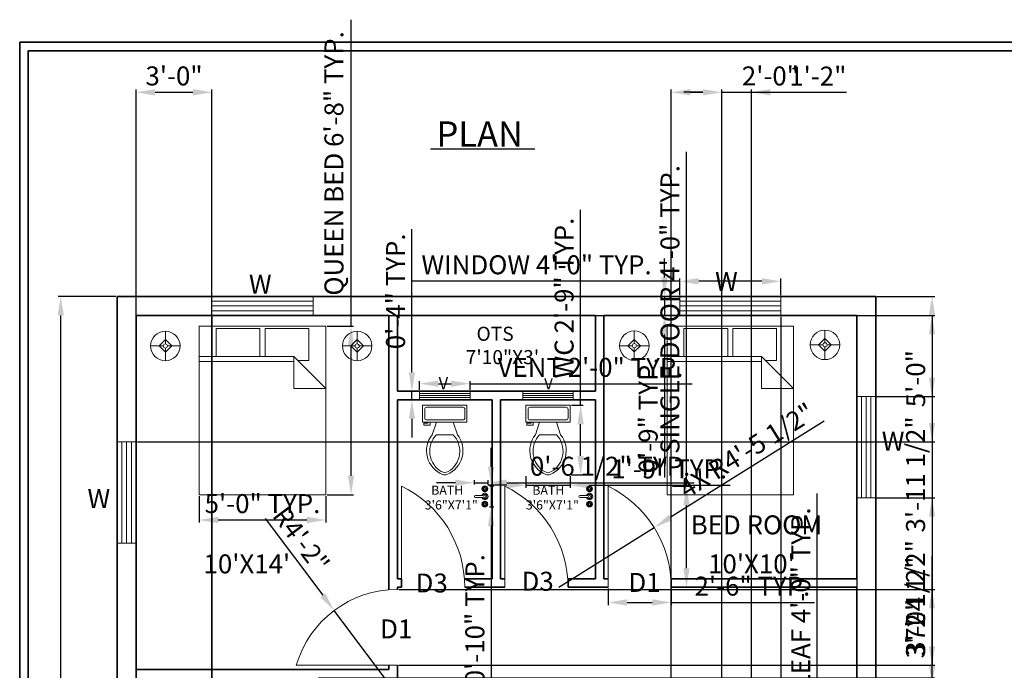
# Model space of a CAD drawing. Units: inches. Extents: x 2436 to 3928, y 1526 to 2149.
# Tile 4 of 6: x 2436 to 2903, y 1840 to 2149. Entities that reach past the tile are written whole.
import ezdxf

# ---------------------------------------------------------------- set-up
doc = ezdxf.new("R2010")
doc.units = ezdxf.units.IN
for name, color, linetype, lineweight in [('A-AREA-IDEN', 152, 'Continuous', 18), ('A-DOOR', 4, 'Continuous', 18), ('A-DOOR-TEXT', 30, 'Continuous', 18), ('A-FLOR-FIXT', 9, 'Continuous', 18), ('A-FURN', 8, 'Continuous', 18), ('A-GLAZ', 2, 'Continuous', 18), ('A-GLAZ-TEXT', 114, 'Continuous', 18), ('A-WALL', 7, 'Continuous', 35), ('G-ANNO-TEXT', 7, 'Continuous', 25), ('G-ANNO-TTLB', 7, 'Continuous', 35), ('S-ANNO-DIMS', 2, 'Continuous', 18)]:
    doc.layers.add(name, color=color, linetype=linetype, lineweight=lineweight)
doc.styles.get("Standard").update_dxf_attribs({"font": 'arial.ttf'})
doc.dimstyles.new('ISO-25', dxfattribs={"dimtxt": 9, "dimasz": 9, "dimexe": 1.25, "dimexo": 0.625, "dimgap": 2, "dimtad": 1, "dimdec": 1, "dimlunit": 4, "dimtxsty": 'Standard', "dimcen": 2.5, "dimadec": 0, "dimazin": 0, "dimtfac": 1, "dimtdec": 1, "dimtmove": 0, "dimatfit": 3, "dimfxl": 1, "dimarcsym": 0})

# ---------------------------------------------------------------- blocks, each defined once
blk = doc.blocks.new('Bed - Queen')
for p, q in [((0, -80.00003), (0, 0)), ((0, 0), (59.99999, 0)), ((59.99999, 0), (59.99999, -80.00003)), ((7.99999, -1.2), (28.79998, -1.2)), ((7.99999, -14.4), (7.99999, -1.2)), ((28.79998, -1.2), (28.79998, -14.4)), ((31.19999, -1.2), (51.99999, -1.2)), ((31.19999, -14.4), (31.19999, -1.2)), ((51.99999, -1.2), (51.99999, -16.4)), ((0, -14.4), (44.8, -14.4)), ((44.8, -16.8), (0, -16.8)), ((59.99999, -29.6), (44.8, -14.4)), ((44.8, -14.4), (44.8, -29.6)), ((51.99999, -16.4), (46.79936, -16.4)), ((44.8, -29.6), (59.99999, -29.6)), ((59.99999, -80.00003), (0, -80.00003))]:
    blk.add_line(p, q)
blk = doc.blocks.new('Toilet - top')
for p, q in [((9.5, -6), (9.5, -2)), ((-10, -8.5), (-8, -8.5)), ((-10, -9.5), (-10, -8.5)), ((-8, -8.5), (-8, -8)), ((-7, -8), (-7, -9.5)), ((-4, -8), (-6, -14)), ((4, -8), (6, -14)), ((-7, -9.5), (-10, -9.5)), ((4, -14), (-4, -14))]:
    blk.add_line(p, q)
blk.add_lwpolyline([(10.5, -8), (10.5, 0), (-10.5, 0), (-10.5, -8)], close=True)
for points in [[(-9.5, -2), (-9.5, -6)], [(8.5, -1), (-8.5, -1)], [(-8.5, -7), (8.5, -7)]]:
    blk.add_lwpolyline(points)
for centre, radius, start, end in [((-8.62, -1.88), 0.884, 81.8699, 188.1301), ((8.62, -1.88), 0.884, 351.8699, 98.1301), ((-8.62, -6.12), 0.884, 171.8699, 278.1301), ((8.62, -6.12), 0.884, 261.8699, 8.1301), ((3.52, -21.58), 12.17, 141.4691, 247.9714), ((4.2, -21.82), 11.33, 136.3677, 238.9468), ((-3.52, -21.58), 12.17, 292.0284, 38.5307), ((-4.2, -21.82), 11.33, 301.053, 43.6321), ((0, -27.88), 4, 245.7318, 294.2682), ((0, -29), 4, 254.8605, 285.1395)]:
    blk.add_arc(centre, radius, start, end)
blk = doc.blocks.new('Faucet - Bathroom top')
for p, q in [((-4.107, 0.125), (-4.375, 0.125)), ((-3.75, 0.4788), (-3.75, 0.75)), ((-3.5, 0.482), (-3.5, 0.75)), ((-3.1461, 0.125), (-2.875, 0.125)), ((3.143, 0.125), (2.875, 0.125)), ((3.5, 0.4788), (3.5, 0.75)), ((3.75, 0.482), (3.75, 0.75)), ((4.1039, 0.125), (4.375, 0.125)), ((-4.1039, -0.125), (-4.375, -0.125)), ((-3.75, -0.4821), (-3.75, -0.75)), ((-3.5, -0.4789), (-3.5, -0.75)), ((-3.143, -0.125), (-2.875, -0.125)), ((-0.5, -0.8639), (-0.5, -4.5)), ((0.5, -4.5), (0.5, -0.8631)), ((3.1461, -0.125), (2.875, -0.125)), ((3.5, -0.4821), (3.5, -0.75)), ((3.75, -0.4789), (3.75, -0.75)), ((4.107, -0.125), (4.375, -0.125))]:
    blk.add_line(p, q)
for centre, radius in [((-3.625, 0), 1.375), ((-4.625, 0), 0.2795), ((-3.625, 0), 0.5), ((-3.625, 1), 0.2795), ((-2.625, 0), 0.2795), ((0, 0), 0.5), ((3.625, 0), 1.375), ((2.625, 0), 0.2795), ((3.625, 0), 0.5), ((3.625, 1), 0.2795), ((4.625, 0), 0.2795), ((-3.625, -1), 0.2795), ((3.625, -1), 0.2795)]:
    blk.add_circle(centre, radius)
for centre, radius, start, end in [((-3.625, 0), 1, 105.2407, 164.2093), ((-3.625, 0), 1, 16.44125, 74.07887), ((0, 0), 1.5, 289.6514, 250.3603), ((0, 0), 1, 300.3431, 239.7554), ((3.625, 0), 1, 106.12, 164.0884), ((3.625, 0), 1, 16.23422, 73.90469), ((-3.625, 0), 1, 196.2342, 253.9047), ((-3.625, 0), 1, 286.12, 344.0884), ((0, -4.5), 0.5, 180, 0), ((3.625, 0), 1, 196.4413, 254.0789), ((3.625, 0), 1, 285.2407, 344.2093)]:
    blk.add_arc(centre, radius, start, end)
blk = doc.blocks.new('Lamp - Table')
for p, q in [((0, 7), (0, 1)), ((-1, 0), (-7, 0)), ((0, 3), (-3, 0)), ((-3, 0), (0, -3)), ((3, 0), (0, 3)), ((0, -3), (3, 0)), ((1, 0), (7, 0)), ((0, -1), (0, -7))]:
    blk.add_line(p, q)
for radius in [7, 1]:
    blk.add_circle((0, 0), radius)
blk = doc.blocks.new('WIN-48x9-PLAN')
for p, q in [((0, 0), (0, 9)), ((0, 6.75), (48, 6.75)), ((48, 0), (48, 9)), ((0, 4.5), (48, 4.5)), ((0, 2.25), (48, 2.25))]:
    blk.add_line(p, q)
blk = doc.blocks.new('VENT-24x4-PLAN')
for p, q in [((0, 0), (0, 4)), ((0, 3), (24, 3)), ((0, 2), (24, 2)), ((0, 1), (24, 1)), ((24, 0), (24, 4))]:
    blk.add_line(p, q)
blk = doc.blocks.new('DOOR-SINGLE-30-PLAN')
blk.add_line((0, 0), (0, 48))
blk.add_arc((-23.4, 0), 53.4, 0, 64.0108)
blk = doc.blocks.new('*D34')
at = {"layer": 'Defpoints', "color": 0, "transparency": 16777216}
for p in [(2749.24, 2024.99), (2749.24, 2017.79), (2797.24, 2017.79)]:
    blk.add_point(p, dxfattribs=at)
at = {"layer": 'S-ANNO-DIMS', "color": 0, "lineweight": -2, "transparency": 16777216}
for p, q in [((2749.24, 2024.99), (2622.35, 2024.99)), ((2749.24, 2018.41), (2749.24, 2026.24)), ((2788.24, 2024.99), (2758.24, 2024.99)), ((2797.24, 2018.41), (2797.24, 2026.24))]:
    blk.add_line(p, q, dxfattribs=at)
at = {"layer": 'S-ANNO-DIMS', "color": 0, "transparency": 16777216}
for points in [[(2758.24, 2026.49), (2758.24, 2023.49), (2749.24, 2024.99)], [(2788.24, 2026.49), (2788.24, 2023.49), (2797.24, 2024.99)]]:
    blk.add_solid(points, dxfattribs=at)
at = {"layer": 'S-ANNO-DIMS', "color": 0, "transparency": 16777216, "insert": (2681.29, 2031.65), "char_height": 9, "attachment_point": 5}
blk.add_mtext('WINDOW 4\'-0" TYP.', dxfattribs=at)
blk = doc.blocks.new('*D35')
at = {"layer": 'Defpoints', "color": 0, "transparency": 16777216}
for p in [(2749.24, 2017.79), (2742.04, 2008.79), (2749.24, 2008.79)]:
    blk.add_point(p, dxfattribs=at)
at = {"layer": 'S-ANNO-DIMS', "color": 0, "lineweight": -2, "transparency": 16777216}
for p, q in [((2742.04, 2026.79), (2742.04, 2035.79)), ((2748.61, 2017.79), (2740.79, 2017.79)), ((2742.04, 2017.79), (2742.04, 2008.79)), ((2748.61, 2008.79), (2740.79, 2008.79)), ((2742.04, 1999.79), (2742.04, 1931.93))]:
    blk.add_line(p, q, dxfattribs=at)
at = {"layer": 'S-ANNO-DIMS', "color": 0, "transparency": 16777216}
for points in [[(2740.54, 2026.79), (2743.54, 2026.79), (2742.04, 2017.79)], [(2740.54, 1999.79), (2743.54, 1999.79), (2742.04, 2008.79)]]:
    blk.add_solid(points, dxfattribs=at)
at = {"layer": 'S-ANNO-DIMS', "color": 0, "transparency": 16777216, "insert": (2735.44, 1961.36), "char_height": 9, "attachment_point": 5, "rotation": 90}
blk.add_mtext('0\'-9" TYP.', dxfattribs=at)
blk = doc.blocks.new('*D36')
at = {"layer": 'Defpoints', "color": 0, "transparency": 16777216}
for p in [(2745.24, 1927.79), (2752.44, 1927.79), (2745.24, 1879.79)]:
    blk.add_point(p, dxfattribs=at)
at = {"layer": 'S-ANNO-DIMS', "color": 0, "lineweight": -2, "transparency": 16777216}
for p, q in [((2752.44, 1927.79), (2752.44, 2086.43)), ((2745.86, 1927.79), (2753.69, 1927.79)), ((2752.44, 1888.79), (2752.44, 1918.79)), ((2745.86, 1879.79), (2753.69, 1879.79))]:
    blk.add_line(p, q, dxfattribs=at)
at = {"layer": 'S-ANNO-DIMS', "color": 0, "transparency": 16777216}
for points in [[(2750.94, 1918.79), (2753.94, 1918.79), (2752.44, 1927.79)], [(2750.94, 1888.79), (2753.94, 1888.79), (2752.44, 1879.79)]]:
    blk.add_solid(points, dxfattribs=at)
at = {"layer": 'S-ANNO-DIMS', "color": 0, "transparency": 16777216, "insert": (2745.78, 2011.61), "char_height": 9, "attachment_point": 5, "rotation": 90}
blk.add_mtext('SINGLE DOOR 4\'-0" TYP.', dxfattribs=at)
blk = doc.blocks.new('*D37')
at = {"layer": 'Defpoints', "color": 0, "transparency": 16777216}
for p in [(2715.24, 1879.79), (2745.24, 1879.79), (2745.24, 1872.59)]:
    blk.add_point(p, dxfattribs=at)
at = {"layer": 'S-ANNO-DIMS', "color": 0, "lineweight": -2, "transparency": 16777216}
for p, q in [((2715.24, 1879.16), (2715.24, 1871.34)), ((2745.24, 1879.16), (2745.24, 1871.34)), ((2724.24, 1872.59), (2736.24, 1872.59)), ((2745.24, 1872.59), (2813.25, 1872.59))]:
    blk.add_line(p, q, dxfattribs=at)
at = {"layer": 'S-ANNO-DIMS', "color": 0, "transparency": 16777216}
for points in [[(2724.24, 1874.09), (2724.24, 1871.09), (2715.24, 1872.59)], [(2736.24, 1874.09), (2736.24, 1871.09), (2745.24, 1872.59)]]:
    blk.add_solid(points, dxfattribs=at)
at = {"layer": 'S-ANNO-DIMS', "color": 0, "transparency": 16777216, "insert": (2783.74, 1879.18), "char_height": 9, "attachment_point": 5}
blk.add_mtext('2\'-6" TYP.', dxfattribs=at)
blk = doc.blocks.new('*D38')
at = {"layer": 'Defpoints', "color": 0, "transparency": 16777216}
for p in [(2581.24, 2003.73), (2593.24, 2003.73), (2581.24, 1923.73)]:
    blk.add_point(p, dxfattribs=at)
at = {"layer": 'S-ANNO-DIMS', "color": 0, "lineweight": -2, "transparency": 16777216}
for p, q in [((2593.24, 2003.73), (2593.24, 2149.12)), ((2581.86, 2003.73), (2594.49, 2003.73)), ((2593.24, 1932.73), (2593.24, 1994.73)), ((2581.86, 1923.73), (2594.49, 1923.73))]:
    blk.add_line(p, q, dxfattribs=at)
at = {"layer": 'S-ANNO-DIMS', "color": 0, "transparency": 16777216}
for points in [[(2591.74, 1994.73), (2594.74, 1994.73), (2593.24, 2003.73)], [(2591.74, 1932.73), (2594.74, 1932.73), (2593.24, 1923.73)]]:
    blk.add_solid(points, dxfattribs=at)
at = {"layer": 'S-ANNO-DIMS', "color": 0, "transparency": 16777216, "insert": (2586.31, 2080.92), "char_height": 9, "attachment_point": 5, "rotation": 90}
blk.add_mtext('QUEEN BED 6\'-8" TYP.', dxfattribs=at)
blk = doc.blocks.new('*D39')
at = {"layer": 'Defpoints', "color": 0, "transparency": 16777216}
for p in [(2521.24, 1923.73), (2581.24, 1923.73), (2581.24, 1911.73)]:
    blk.add_point(p, dxfattribs=at)
at = {"layer": 'S-ANNO-DIMS', "color": 0, "lineweight": -2, "transparency": 16777216}
for p, q in [((2521.24, 1923.1), (2521.24, 1910.48)), ((2581.24, 1923.1), (2581.24, 1910.48)), ((2530.24, 1911.73), (2572.24, 1911.73))]:
    blk.add_line(p, q, dxfattribs=at)
at = {"layer": 'S-ANNO-DIMS', "color": 0, "transparency": 16777216}
for points in [[(2530.24, 1913.23), (2530.24, 1910.23), (2521.24, 1911.73)], [(2572.24, 1913.23), (2572.24, 1910.23), (2581.24, 1911.73)]]:
    blk.add_solid(points, dxfattribs=at)
at = {"layer": 'S-ANNO-DIMS', "color": 0, "transparency": 16777216, "insert": (2551.24, 1918.32), "char_height": 9, "attachment_point": 5}
blk.add_mtext('5\'-0" TYP.', dxfattribs=at)
blk = doc.blocks.new('*D40')
at = {"layer": 'Defpoints', "color": 0, "transparency": 16777216}
for p in [(2697.24, 1966.19), (2702.2, 1966.19), (2697.24, 1933.15)]:
    blk.add_point(p, dxfattribs=at)
at = {"layer": 'S-ANNO-DIMS', "color": 0, "lineweight": -2, "transparency": 16777216}
for p, q in [((2702.2, 1966.19), (2702.2, 2058.86)), ((2697.86, 1966.19), (2703.45, 1966.19)), ((2702.2, 1942.15), (2702.2, 1957.19)), ((2697.86, 1933.15), (2703.45, 1933.15))]:
    blk.add_line(p, q, dxfattribs=at)
at = {"layer": 'S-ANNO-DIMS', "color": 0, "transparency": 16777216}
for points in [[(2700.7, 1957.19), (2703.7, 1957.19), (2702.2, 1966.19)], [(2700.7, 1942.15), (2703.7, 1942.15), (2702.2, 1933.15)]]:
    blk.add_solid(points, dxfattribs=at)
at = {"layer": 'S-ANNO-DIMS', "color": 0, "transparency": 16777216, "insert": (2695.54, 2017.03), "char_height": 9, "attachment_point": 5, "rotation": 90}
blk.add_mtext('WC 2\'-9" TYP.', dxfattribs=at)
blk = doc.blocks.new('*D41')
at = {"layer": 'Defpoints', "color": 0, "transparency": 16777216}
for p in [(2676.24, 1933.15), (2697.24, 1933.15), (2697.24, 1928.19)]:
    blk.add_point(p, dxfattribs=at)
at = {"layer": 'S-ANNO-DIMS', "color": 0, "lineweight": -2, "transparency": 16777216}
for p, q in [((2676.24, 1932.52), (2676.24, 1926.94)), ((2697.24, 1932.52), (2697.24, 1926.94)), ((2667.24, 1928.19), (2658.24, 1928.19)), ((2676.24, 1928.19), (2697.24, 1928.19)), ((2706.24, 1928.19), (2773.25, 1928.19))]:
    blk.add_line(p, q, dxfattribs=at)
at = {"layer": 'S-ANNO-DIMS', "color": 0, "transparency": 16777216}
for points in [[(2667.24, 1929.69), (2667.24, 1926.69), (2676.24, 1928.19)], [(2706.24, 1929.69), (2706.24, 1926.69), (2697.24, 1928.19)]]:
    blk.add_solid(points, dxfattribs=at)
at = {"layer": 'S-ANNO-DIMS', "color": 0, "transparency": 16777216, "insert": (2744.24, 1934.78), "char_height": 9, "attachment_point": 5}
blk.add_mtext('1\'-9" TYP.', dxfattribs=at)
blk = doc.blocks.new('*D42')
at = {"layer": 'Defpoints', "color": 0, "transparency": 16777216}
for p in [(2658.27, 1927.9), (2658.27, 1917.9), (2659.77, 1917.9)]:
    blk.add_point(p, dxfattribs=at)
at = {"layer": 'S-ANNO-DIMS', "color": 0, "lineweight": -2, "transparency": 16777216}
for p, q in [((2659.77, 1936.9), (2659.77, 1945.9)), ((2658.9, 1927.9), (2661.02, 1927.9)), ((2659.77, 1927.9), (2659.77, 1917.9)), ((2658.9, 1917.9), (2661.02, 1917.9)), ((2659.77, 1908.9), (2659.77, 1769.48))]:
    blk.add_line(p, q, dxfattribs=at)
at = {"layer": 'S-ANNO-DIMS', "color": 0, "transparency": 16777216}
for points in [[(2658.27, 1936.9), (2661.27, 1936.9), (2659.77, 1927.9)], [(2658.27, 1908.9), (2661.27, 1908.9), (2659.77, 1917.9)]]:
    blk.add_solid(points, dxfattribs=at)
at = {"layer": 'S-ANNO-DIMS', "color": 0, "transparency": 16777216, "insert": (2653.18, 1834.69), "char_height": 9, "attachment_point": 5, "rotation": 90}
blk.add_mtext('BATH TAP 0\'-10" TYP.', dxfattribs=at)
blk = doc.blocks.new('*D43')
at = {"layer": 'Defpoints', "color": 0, "transparency": 16777216}
for p in [(2651.77, 1927.9), (2658.27, 1929.4), (2658.27, 1927.9)]:
    blk.add_point(p, dxfattribs=at)
at = {"layer": 'S-ANNO-DIMS', "color": 0, "lineweight": -2, "transparency": 16777216}
for p, q in [((2651.77, 1928.53), (2651.77, 1930.65)), ((2658.27, 1928.53), (2658.27, 1930.65)), ((2642.77, 1929.4), (2633.77, 1929.4)), ((2651.77, 1929.4), (2658.27, 1929.4)), ((2667.27, 1929.4), (2756.1, 1929.4))]:
    blk.add_line(p, q, dxfattribs=at)
at = {"layer": 'S-ANNO-DIMS', "color": 0, "transparency": 16777216}
for points in [[(2642.77, 1930.9), (2642.77, 1927.9), (2651.77, 1929.4)], [(2667.27, 1930.9), (2667.27, 1927.9), (2658.27, 1929.4)]]:
    blk.add_solid(points, dxfattribs=at)
at = {"layer": 'S-ANNO-DIMS', "color": 0, "transparency": 16777216, "insert": (2716.19, 1936.06), "char_height": 9, "attachment_point": 5}
blk.add_mtext('0\'-6 1/2" TYP.', dxfattribs=at)
blk = doc.blocks.new('*D44')
at = {"layer": 'Defpoints', "color": 0, "transparency": 16777216}
for p in [(2625.74, 1972.79), (2649.74, 1976.39), (2649.74, 1972.79)]:
    blk.add_point(p, dxfattribs=at)
at = {"layer": 'S-ANNO-DIMS', "color": 0, "lineweight": -2, "transparency": 16777216}
for p, q in [((2625.74, 1973.41), (2625.74, 1977.64)), ((2649.74, 1973.41), (2649.74, 1977.64)), ((2634.74, 1976.39), (2640.74, 1976.39)), ((2649.74, 1976.39), (2755.09, 1976.39))]:
    blk.add_line(p, q, dxfattribs=at)
at = {"layer": 'S-ANNO-DIMS', "color": 0, "transparency": 16777216}
for points in [[(2634.74, 1977.89), (2634.74, 1974.89), (2625.74, 1976.39)], [(2640.74, 1977.89), (2640.74, 1974.89), (2649.74, 1976.39)]]:
    blk.add_solid(points, dxfattribs=at)
at = {"layer": 'S-ANNO-DIMS', "color": 0, "transparency": 16777216, "insert": (2706.91, 1982.98), "char_height": 9, "attachment_point": 5}
blk.add_mtext('VENT 2\'-0" TYP.', dxfattribs=at)
blk = doc.blocks.new('*D45')
at = {"layer": 'Defpoints', "color": 0, "transparency": 16777216}
for p in [(2622.14, 1972.79), (2625.74, 1972.79), (2625.74, 1968.79)]:
    blk.add_point(p, dxfattribs=at)
at = {"layer": 'S-ANNO-DIMS', "color": 0, "lineweight": -2, "transparency": 16777216}
for p, q in [((2622.14, 1981.79), (2622.14, 2049.65)), ((2625.11, 1972.79), (2620.89, 1972.79)), ((2622.14, 1968.79), (2622.14, 1972.79)), ((2625.11, 1968.79), (2620.89, 1968.79)), ((2622.14, 1959.79), (2622.14, 1950.79))]:
    blk.add_line(p, q, dxfattribs=at)
at = {"layer": 'S-ANNO-DIMS', "color": 0, "transparency": 16777216}
for points in [[(2620.64, 1981.79), (2623.64, 1981.79), (2622.14, 1972.79)], [(2620.64, 1959.79), (2623.64, 1959.79), (2622.14, 1968.79)]]:
    blk.add_solid(points, dxfattribs=at)
at = {"layer": 'S-ANNO-DIMS', "color": 0, "transparency": 16777216, "insert": (2615.54, 2020.22), "char_height": 9, "attachment_point": 5, "rotation": 90}
blk.add_mtext('0\'-4" TYP.', dxfattribs=at)
blk = doc.blocks.new('*D46')
at = {"layer": 'Defpoints', "color": 0, "transparency": 16777216}
for p in [(2807.24, 1775.79), (2814.44, 1775.79), (2807.24, 1727.79)]:
    blk.add_point(p, dxfattribs=at)
at = {"layer": 'S-ANNO-DIMS', "color": 0, "lineweight": -2, "transparency": 16777216}
for p, q in [((2814.44, 1775.79), (2814.44, 1924.22)), ((2807.86, 1775.79), (2815.69, 1775.79)), ((2814.44, 1736.79), (2814.44, 1766.79)), ((2807.86, 1727.79), (2815.69, 1727.79))]:
    blk.add_line(p, q, dxfattribs=at)
at = {"layer": 'S-ANNO-DIMS', "color": 0, "transparency": 16777216}
for points in [[(2812.94, 1766.79), (2815.94, 1766.79), (2814.44, 1775.79)], [(2812.94, 1736.79), (2815.94, 1736.79), (2814.44, 1727.79)]]:
    blk.add_solid(points, dxfattribs=at)
at = {"layer": 'S-ANNO-DIMS', "color": 0, "transparency": 16777216, "insert": (2807.84, 1854.5), "char_height": 9, "attachment_point": 5, "rotation": 90}
blk.add_mtext('ENTRY LEAF 4\'-0" TYP.', dxfattribs=at)
blk = doc.blocks.new('*D57')
at = {"layer": 'Defpoints', "color": 0, "transparency": 16777216}
for p in [(2455.49, 2017.79), (2482.24, 2017.79), (2482.24, 1577.79)]:
    blk.add_point(p, dxfattribs=at)
at = {"layer": 'S-ANNO-DIMS', "color": 0, "lineweight": -2, "transparency": 16777216}
for p, q in [((2481.61, 2017.79), (2454.24, 2017.79)), ((2455.49, 1586.79), (2455.49, 2008.79)), ((2481.61, 1577.79), (2454.24, 1577.79))]:
    blk.add_line(p, q, dxfattribs=at)
at = {"layer": 'S-ANNO-DIMS', "color": 0, "transparency": 16777216}
for points in [[(2453.99, 2008.79), (2456.99, 2008.79), (2455.49, 2017.79)], [(2453.99, 1586.79), (2456.99, 1586.79), (2455.49, 1577.79)]]:
    blk.add_solid(points, dxfattribs=at)
at = {"layer": 'S-ANNO-DIMS', "color": 0, "transparency": 16777216, "insert": (2448.89, 1797.79), "char_height": 9, "attachment_point": 5, "rotation": 90}
blk.add_mtext('36\'-8"', dxfattribs=at)
blk = doc.blocks.new('*D58')
at = {"layer": 'Defpoints', "color": 0, "transparency": 16777216}
for p in [(2491.24, 2008.79), (2527.24, 2008.79), (2527.24, 1551.04)]:
    blk.add_point(p, dxfattribs=at)
at = {"layer": 'S-ANNO-DIMS', "color": 0, "lineweight": -2, "transparency": 16777216}
for p, q in [((2491.24, 2008.16), (2491.24, 1549.79)), ((2527.24, 2008.16), (2527.24, 1549.79)), ((2500.24, 1551.04), (2518.24, 1551.04))]:
    blk.add_line(p, q, dxfattribs=at)
at = {"layer": 'S-ANNO-DIMS', "color": 0, "transparency": 16777216}
for points in [[(2500.24, 1552.54), (2500.24, 1549.54), (2491.24, 1551.04)], [(2518.24, 1552.54), (2518.24, 1549.54), (2527.24, 1551.04)]]:
    blk.add_solid(points, dxfattribs=at)
at = {"layer": 'S-ANNO-DIMS', "color": 0, "transparency": 16777216, "insert": (2509.24, 1557.64), "char_height": 9, "attachment_point": 5}
blk.add_mtext('3\'-0"', dxfattribs=at)
blk = doc.blocks.new('*D59')
at = {"layer": 'Defpoints', "color": 0, "transparency": 16777216}
for p in [(2797.24, 2008.79), (2833.24, 2008.79), (2833.24, 1551.04)]:
    blk.add_point(p, dxfattribs=at)
at = {"layer": 'S-ANNO-DIMS', "color": 0, "lineweight": -2, "transparency": 16777216}
for p, q in [((2797.24, 2008.16), (2797.24, 1549.79)), ((2833.24, 2008.16), (2833.24, 1549.79)), ((2806.24, 1551.04), (2824.24, 1551.04))]:
    blk.add_line(p, q, dxfattribs=at)
at = {"layer": 'S-ANNO-DIMS', "color": 0, "transparency": 16777216}
for points in [[(2806.24, 1552.54), (2806.24, 1549.54), (2797.24, 1551.04)], [(2824.24, 1552.54), (2824.24, 1549.54), (2833.24, 1551.04)]]:
    blk.add_solid(points, dxfattribs=at)
at = {"layer": 'S-ANNO-DIMS', "color": 0, "transparency": 16777216, "insert": (2815.24, 1557.64), "char_height": 9, "attachment_point": 5}
blk.add_mtext('3\'-0"', dxfattribs=at)
blk = doc.blocks.new('*D60')
at = {"layer": 'Defpoints', "color": 0, "transparency": 16777216}
for p in [(2842.24, 2017.79), (2842.24, 1970.29), (2868.99, 1970.29)]:
    blk.add_point(p, dxfattribs=at)
at = {"layer": 'S-ANNO-DIMS', "color": 0, "lineweight": -2, "transparency": 16777216}
for p, q in [((2842.86, 2017.79), (2870.24, 2017.79)), ((2868.99, 2008.79), (2868.99, 1979.29)), ((2842.86, 1970.29), (2870.24, 1970.29)), ((2868.99, 1970.29), (2868.99, 1905.41))]:
    blk.add_line(p, q, dxfattribs=at)
at = {"layer": 'S-ANNO-DIMS', "color": 0, "transparency": 16777216}
for points in [[(2867.49, 2008.79), (2870.49, 2008.79), (2868.99, 2017.79)], [(2867.49, 1979.29), (2870.49, 1979.29), (2868.99, 1970.29)]]:
    blk.add_solid(points, dxfattribs=at)
at = {"layer": 'S-ANNO-DIMS', "color": 0, "transparency": 16777216, "insert": (2862.33, 1933.35), "char_height": 9, "attachment_point": 5, "rotation": 90}
blk.add_mtext('3\'-11 1/2"', dxfattribs=at)
blk = doc.blocks.new('*D61')
at = {"layer": 'Defpoints', "color": 0, "transparency": 16777216}
for p in [(2842.24, 1922.29), (2842.24, 1833.79), (2868.99, 1833.79)]:
    blk.add_point(p, dxfattribs=at)
at = {"layer": 'S-ANNO-DIMS', "color": 0, "lineweight": -2, "transparency": 16777216}
for p, q in [((2842.86, 1922.29), (2870.24, 1922.29)), ((2868.99, 1913.29), (2868.99, 1842.79)), ((2842.86, 1833.79), (2870.24, 1833.79))]:
    blk.add_line(p, q, dxfattribs=at)
at = {"layer": 'S-ANNO-DIMS', "color": 0, "transparency": 16777216}
for points in [[(2867.49, 1913.29), (2870.49, 1913.29), (2868.99, 1922.29)], [(2867.49, 1842.79), (2870.49, 1842.79), (2868.99, 1833.79)]]:
    blk.add_solid(points, dxfattribs=at)
at = {"layer": 'S-ANNO-DIMS', "color": 0, "transparency": 16777216, "insert": (2862.33, 1878.04), "char_height": 9, "attachment_point": 5, "rotation": 90}
blk.add_mtext('7\'-4 1/2"', dxfattribs=at)
blk = doc.blocks.new('*D62')
at = {"layer": 'Defpoints', "color": 0, "transparency": 16777216}
for p in [(2491.24, 2008.79), (2491.24, 1948.79), (2868.99, 1948.79)]:
    blk.add_point(p, dxfattribs=at)
at = {"layer": 'S-ANNO-DIMS', "color": 0, "lineweight": -2, "transparency": 16777216}
for p, q in [((2491.86, 2008.79), (2870.24, 2008.79)), ((2868.99, 1999.79), (2868.99, 1957.79)), ((2491.86, 1948.79), (2870.24, 1948.79))]:
    blk.add_line(p, q, dxfattribs=at)
at = {"layer": 'S-ANNO-DIMS', "color": 0, "transparency": 16777216}
for points in [[(2867.49, 1999.79), (2870.49, 1999.79), (2868.99, 2008.79)], [(2867.49, 1957.79), (2870.49, 1957.79), (2868.99, 1948.79)]]:
    blk.add_solid(points, dxfattribs=at)
at = {"layer": 'S-ANNO-DIMS', "color": 0, "transparency": 16777216, "insert": (2862.39, 1978.79), "char_height": 9, "attachment_point": 5, "rotation": 90}
blk.add_mtext('5\'-0"', dxfattribs=at)
blk = doc.blocks.new('*D64')
at = {"layer": 'Defpoints', "color": 0, "transparency": 16777216}
for p in [(2527.24, 2114.67), (2491.24, 1603.79), (2527.24, 1603.79)]:
    blk.add_point(p, dxfattribs=at)
at = {"layer": 'S-ANNO-DIMS', "color": 0, "lineweight": -2, "transparency": 16777216}
for p, q in [((2491.24, 1604.41), (2491.24, 2115.92)), ((2500.24, 2114.67), (2518.24, 2114.67)), ((2527.24, 1604.41), (2527.24, 2115.92))]:
    blk.add_line(p, q, dxfattribs=at)
at = {"layer": 'S-ANNO-DIMS', "color": 0, "transparency": 16777216}
for points in [[(2500.24, 2116.17), (2500.24, 2113.17), (2491.24, 2114.67)], [(2518.24, 2116.17), (2518.24, 2113.17), (2527.24, 2114.67)]]:
    blk.add_solid(points, dxfattribs=at)
at = {"layer": 'S-ANNO-DIMS', "color": 0, "transparency": 16777216, "insert": (2509.24, 2121.27), "char_height": 9, "attachment_point": 5}
blk.add_mtext('3\'-0"', dxfattribs=at)
blk = doc.blocks.new('*D68')
at = {"layer": 'Defpoints', "color": 0, "transparency": 16777216}
for p in [(2769.24, 2114.67), (2745.24, 1739.79), (2769.24, 1739.79)]:
    blk.add_point(p, dxfattribs=at)
at = {"layer": 'S-ANNO-DIMS', "color": 0, "lineweight": -2, "transparency": 16777216}
for p, q in [((2745.24, 1740.41), (2745.24, 2115.92)), ((2754.24, 2114.67), (2760.24, 2114.67)), ((2769.24, 1740.41), (2769.24, 2115.92)), ((2769.24, 2114.67), (2806.32, 2114.67))]:
    blk.add_line(p, q, dxfattribs=at)
at = {"layer": 'S-ANNO-DIMS', "color": 0, "transparency": 16777216}
for points in [[(2754.24, 2116.17), (2754.24, 2113.17), (2745.24, 2114.67)], [(2760.24, 2116.17), (2760.24, 2113.17), (2769.24, 2114.67)]]:
    blk.add_solid(points, dxfattribs=at)
at = {"layer": 'S-ANNO-DIMS', "color": 0, "transparency": 16777216, "insert": (2792.28, 2121.26), "char_height": 9, "attachment_point": 5}
blk.add_mtext('2\'-0"', dxfattribs=at)
blk = doc.blocks.new('*D69')
at = {"layer": 'Defpoints', "color": 0, "transparency": 16777216}
for p in [(2783.24, 2114.67), (2769.24, 1739.79), (2783.24, 1739.79)]:
    blk.add_point(p, dxfattribs=at)
at = {"layer": 'S-ANNO-DIMS', "color": 0, "lineweight": -2, "transparency": 16777216}
for p, q in [((2760.24, 2114.67), (2751.24, 2114.67)), ((2769.24, 1740.41), (2769.24, 2115.92)), ((2769.24, 2114.67), (2783.24, 2114.67)), ((2783.24, 1740.41), (2783.24, 2115.92)), ((2792.24, 2114.67), (2828.32, 2114.67))]:
    blk.add_line(p, q, dxfattribs=at)
at = {"layer": 'S-ANNO-DIMS', "color": 0, "transparency": 16777216}
for points in [[(2760.24, 2116.17), (2760.24, 2113.17), (2769.24, 2114.67)], [(2792.24, 2116.17), (2792.24, 2113.17), (2783.24, 2114.67)]]:
    blk.add_solid(points, dxfattribs=at)
at = {"layer": 'S-ANNO-DIMS', "color": 0, "transparency": 16777216, "insert": (2814.78, 2121.19), "char_height": 9, "attachment_point": 5}
blk.add_mtext('1\'-2"', dxfattribs=at)
blk = doc.blocks.new('*D70')
at = {"layer": 'Defpoints', "color": 0, "transparency": 16777216}
for p in [(2615.24, 1878.79), (2868.99, 1878.79), (2615.24, 1842.79)]:
    blk.add_point(p, dxfattribs=at)
at = {"layer": 'S-ANNO-DIMS', "color": 0, "lineweight": -2, "transparency": 16777216}
for p, q in [((2615.86, 1878.79), (2870.24, 1878.79)), ((2868.99, 1851.79), (2868.99, 1869.79)), ((2615.86, 1842.79), (2870.24, 1842.79))]:
    blk.add_line(p, q, dxfattribs=at)
at = {"layer": 'S-ANNO-DIMS', "color": 0, "transparency": 16777216}
for points in [[(2867.49, 1869.79), (2870.49, 1869.79), (2868.99, 1878.79)], [(2867.49, 1851.79), (2870.49, 1851.79), (2868.99, 1842.79)]]:
    blk.add_solid(points, dxfattribs=at)
at = {"layer": 'S-ANNO-DIMS', "color": 0, "transparency": 16777216, "insert": (2862.39, 1860.79), "char_height": 9, "attachment_point": 5, "rotation": 90}
blk.add_mtext('3\'-0"', dxfattribs=at)
blk = doc.blocks.new('*D71')
at = {"layer": 'Defpoints', "color": 0, "transparency": 16777216}
for p in [(2577.24, 1836.79), (2868.99, 1836.79), (2577.24, 1798.29)]:
    blk.add_point(p, dxfattribs=at)
at = {"layer": 'S-ANNO-DIMS', "color": 0, "lineweight": -2, "transparency": 16777216}
for p, q in [((2868.99, 1836.79), (2868.99, 1894.68)), ((2577.86, 1836.79), (2870.24, 1836.79)), ((2868.99, 1807.29), (2868.99, 1827.79)), ((2577.86, 1798.29), (2870.24, 1798.29))]:
    blk.add_line(p, q, dxfattribs=at)
at = {"layer": 'S-ANNO-DIMS', "color": 0, "transparency": 16777216}
for points in [[(2867.49, 1827.79), (2870.49, 1827.79), (2868.99, 1836.79)], [(2867.49, 1807.29), (2870.49, 1807.29), (2868.99, 1798.29)]]:
    blk.add_solid(points, dxfattribs=at)
at = {"layer": 'S-ANNO-DIMS', "color": 0, "transparency": 16777216, "insert": (2862.33, 1870.23), "char_height": 9, "attachment_point": 5, "rotation": 90}
blk.add_mtext('3\'-2 1/2"', dxfattribs=at)
blk = doc.blocks.new('*D82')
at = {"layer": 'Defpoints', "color": 0, "transparency": 16777216}
for p in [(2737.12, 1908.09), (2691.84, 1879.79)]:
    blk.add_point(p, dxfattribs=at)
at = {"layer": 'S-ANNO-DIMS', "color": 0, "lineweight": -2, "transparency": 16777216}
for p, q in [((2817.86, 1958.55), (2744.75, 1912.86)), ((2691.84, 1879.79), (2737.12, 1908.09))]:
    blk.add_line(p, q, dxfattribs=at)
at = {"layer": 'S-ANNO-DIMS', "color": 0, "transparency": 16777216}
blk.add_solid([(2743.96, 1914.13), (2745.55, 1911.59), (2737.12, 1908.09)], dxfattribs=at)
at = {"layer": 'S-ANNO-DIMS', "color": 0, "transparency": 16777216, "insert": (2781.6, 1943.73), "char_height": 9, "attachment_point": 5, "rotation": 32.0053}
blk.add_mtext('4X R4\'-5 1/2"', dxfattribs=at)
blk = doc.blocks.new('*D83')
at = {"layer": 'Defpoints', "color": 0, "transparency": 16777216}
for p in [(2585.24, 1868.79), (2615.24, 1828.79)]:
    blk.add_point(p, dxfattribs=at)
at = {"layer": 'S-ANNO-DIMS', "color": 0, "lineweight": -2, "transparency": 16777216}
for p, q in [((2552.51, 1912.42), (2579.84, 1875.99)), ((2615.24, 1828.79), (2585.24, 1868.79))]:
    blk.add_line(p, q, dxfattribs=at)
at = {"layer": 'S-ANNO-DIMS', "color": 0, "transparency": 16777216}
blk.add_solid([(2581.04, 1876.89), (2578.64, 1875.09), (2585.24, 1868.79)], dxfattribs=at)
at = {"layer": 'S-ANNO-DIMS', "color": 0, "transparency": 16777216, "insert": (2568.69, 1901.72), "char_height": 9, "attachment_point": 5, "rotation": 306.8705}
blk.add_mtext('R4\'-2"', dxfattribs=at)

msp = doc.modelspace()

# ---------------------------------------------------------------- linework, layer by layer
at = {"layer": 'A-DOOR'}
msp.add_line((2567.24, 1842.79), (2615.24, 1842.79), dxfattribs=at)
msp.add_arc((2615.24, 1828.79), 50, 90, 163.7398, dxfattribs=at)
at = {"layer": 'A-WALL'}
for p, q in [((2482.24, 2017.79), (2611.24, 2017.79)), ((2482.24, 2017.79), (2842.24, 2017.79)), ((2482.24, 1577.79), (2482.24, 2017.79)), ((2611.24, 2017.79), (2615.24, 2017.79)), ((2615.24, 2017.79), (2709.24, 2017.79)), ((2709.24, 2017.79), (2713.24, 2017.79)), ((2833.24, 2017.79), (2842.24, 2017.79)), ((2842.24, 2017.79), (2842.24, 2008.79)), ((2842.24, 2017.79), (2842.24, 1585.79)), ((2491.24, 2008.79), (2611.24, 2008.79)), ((2491.24, 1840.79), (2491.24, 2008.79)), ((2611.24, 1878.63), (2611.24, 2008.79)), ((2615.24, 2008.79), (2709.24, 2008.79)), ((2615.24, 1972.79), (2615.24, 2008.79)), ((2709.24, 1972.79), (2709.24, 2008.79)), ((2713.24, 1883.79), (2713.24, 2008.79)), ((2713.24, 2008.79), (2833.24, 2008.79)), ((2833.24, 1883.79), (2833.24, 2008.79)), ((2842.24, 2008.79), (2842.24, 1888.79)), ((2615.24, 1972.79), (2709.24, 1972.79)), ((2615.24, 1968.79), (2660.24, 1968.79)), ((2615.24, 1883.79), (2615.24, 1968.79)), ((2660.24, 1883.79), (2660.24, 1968.79)), ((2664.24, 1883.79), (2664.24, 1968.79)), ((2664.24, 1968.79), (2709.24, 1968.79)), ((2709.24, 1883.79), (2709.24, 1968.79)), ((2842.24, 1888.79), (2842.24, 1884.79)), ((2615.24, 1883.79), (2617.24, 1883.79)), ((2617.24, 1879.79), (2617.24, 1883.79)), ((2647.09, 1883.79), (2660.24, 1883.79)), ((2664.24, 1883.79), (2666.24, 1883.79)), ((2696.09, 1883.79), (2709.24, 1883.79)), ((2696.24, 1879.79), (2696.24, 1883.79)), ((2713.24, 1883.79), (2715.24, 1883.79)), ((2745.24, 1879.79), (2745.24, 1883.79)), ((2745.24, 1883.79), (2833.24, 1883.79)), ((2615.24, 1879.79), (2617.24, 1879.79)), ((2615.24, 1878.79), (2615.24, 1879.79)), ((2647.24, 1879.79), (2666.24, 1879.79)), ((2696.24, 1879.79), (2715.24, 1879.79)), ((2745.24, 1879.79), (2833.24, 1879.79)), ((2833.24, 1739.79), (2833.24, 1879.79)), ((2611.24, 1840.79), (2611.24, 1842.79)), ((2615.24, 1836.79), (2615.24, 1842.79)), ((2491.24, 1840.79), (2611.24, 1840.79))]:
    msp.add_line(p, q, dxfattribs=at)
at = {"layer": 'G-ANNO-TEXT'}
msp.add_line((2631.03, 2087.92), (2680.51, 2087.92), dxfattribs=at)
at = {"layer": 'G-ANNO-TTLB'}
for points in [[(2436, 2138.4), (3927.51, 2138.4), (3927.51, 1525.6), (2436, 1525.6)], [(2440, 2134.4), (3923.51, 2134.4), (3923.51, 1529.6), (2440, 1529.6)]]:
    msp.add_lwpolyline(points, close=True, dxfattribs=at)

# ---------------------------------------------------------------- block references
at = {"layer": 'A-DOOR'}
for p in [(2617.24, 1879.79), (2666.24, 1879.79), (2715.24, 1879.79)]:
    msp.add_blockref('DOOR-SINGLE-30-PLAN', p, dxfattribs=at)
at = {"layer": 'A-FLOR-FIXT'}
for p in [(2637.74, 1966.19), (2686.74, 1966.19)]:
    msp.add_blockref('Toilet - top', p, dxfattribs=at)
at = {"layer": 'A-FLOR-FIXT', "rotation": 270}
for p in [(2656.77, 1922.9), (2706.44, 1922.9)]:
    msp.add_blockref('Faucet - Bathroom top', p, dxfattribs=at)
at = {"layer": 'A-FURN'}
for name, p in [('Lamp - Table', (2505.14, 1994.3)), ('Bed - Queen', (2521.24, 2003.73)), ('Lamp - Table', (2596.14, 1994.3)), ('Lamp - Table', (2727.68, 1994.44)), ('Bed - Queen', (2743.24, 2003.73)), ('Lamp - Table', (2818.17, 1994.81))]:
    msp.add_blockref(name, p, dxfattribs=at)
at = {"layer": 'A-GLAZ'}
for name, p in [('WIN-48x9-PLAN', (2527.24, 2008.79)), ('VENT-24x4-PLAN', (2625.74, 1968.79)), ('VENT-24x4-PLAN', (2674.74, 1968.79))]:
    msp.add_blockref(name, p, dxfattribs=at)
for p, rotation in [((2797.24, 2017.79), 180), ((2833.24, 1970.29), 270.0000000000039), ((2482.24, 1948.79), 270.0000000000041)]:
    msp.add_blockref('WIN-48x9-PLAN', p, dxfattribs=dict(at, rotation=rotation))

# ---------------------------------------------------------------- texts
at = {"layer": 'A-AREA-IDEN'}
for s, height, p in [('OTS', 6.681, (2652.8, 1996.75)), ('7\'10"X3\'', 6.681, (2647.68, 1985.67)), ('BATH', 4.297, (2631.3, 1923.7)), ('BATH', 4.297, (2679.29, 1923.7)), ('3\'6"X7\'1"', 4.297, (2628.23, 1916.71)), ('3\'6"X7\'1"', 4.297, (2676.21, 1916.71)), ('BED ROOM', 9, (2754.47, 1904.91)), ("   10'X14'", 9, (2515, 1886.38)), ("   10'X10'", 9, (2754.47, 1886.38))]:
    msp.add_text(s, height=height, dxfattribs=at).set_placement(p)
at = {"layer": 'A-DOOR-TEXT'}
for s, p in [('D3', (2623.9, 1877.32)), ('D3', (2674.19, 1878.15)), ('D1', (2724.91, 1877.61)), ('D1', (2607.08, 1855.53))]:
    msp.add_text(s, height=9, dxfattribs=at).set_placement(p)
at = {"layer": 'A-GLAZ-TEXT'}
for s, height, p in [('W', 9, (2544.79, 2019.16)), ('W', 9, (2766.01, 2020.44)), ('V', 5.78, (2634.81, 1973.76)), ('V', 5.25, (2684.92, 1973.73)), ('W', 9, (2845.12, 1944.57)), ('W', 9, (2468.17, 1917.36))]:
    msp.add_text(s, height=height, dxfattribs=at).set_placement(p)
at = {"layer": 'G-ANNO-TEXT'}
msp.add_text('PLAN', height=12, dxfattribs=at).set_placement((2633.81, 2088.86))

# ---------------------------------------------------------------- dimensions: what is measured, and where the dimension line sits
at = {"layer": 'S-ANNO-DIMS'}
for base, p1, p2, angle, text, picture, middle in [((2593.24, 2003.73), (2581.24, 1923.73), (2581.24, 2003.73), 90, 'QUEEN BED <> TYP.', '*D38', (2586.31, 2080.92)), ((2752.44, 1927.79), (2745.24, 1879.79), (2745.24, 1927.79), 90, 'SINGLE DOOR <> TYP.', '*D36', (2745.78, 2011.61)), ((2702.2, 1966.19), (2697.24, 1933.15), (2697.24, 1966.19), 90, 'WC <> TYP.', '*D40', (2695.54, 2017.03)), ((2749.24, 2024.99), (2797.24, 2017.79), (2749.24, 2017.79), 180, 'WINDOW <> TYP.', '*D34', (2681.29, 2031.65)), ((2622.14, 1972.79), (2625.74, 1968.79), (2625.74, 1972.79), 90, '<> TYP.', '*D45', (2615.54, 2020.22)), ((2742.04, 2008.79), (2749.24, 2017.79), (2749.24, 2008.79), 270, '<> TYP.', '*D35', (2735.44, 1961.36)), ((2659.77, 1917.9), (2658.27, 1927.9), (2658.27, 1917.9), 270, 'BATH TAP <> TYP.', '*D42', (2653.18, 1834.69)), ((2814.44, 1775.79), (2807.24, 1727.79), (2807.24, 1775.79), 90, 'ENTRY LEAF <> TYP.', '*D46', (2807.84, 1854.5))]:
    dim = msp.add_linear_dim(base=base, p1=p1, p2=p2, angle=angle, text=text, dimstyle='ISO-25', override={"dimdec": 1, "dimlfac": 1, "dimrnd": 0, "dimzin": 1, "dimdsep": 46, "dimlunit": 4, "dimfrac": 2}, dxfattribs=at)
    dim.commit()
    dim.dimension.update_dxf_attribs({"geometry": picture, "text_midpoint": middle})
for base, p1, p2, picture, middle in [((2527.24, 2114.67), (2491.24, 1603.79), (2527.24, 1603.79), '*D64', (2509.24, 2121.27)), ((2769.24, 2114.67), (2745.24, 1739.79), (2769.24, 1739.79), '*D68', (2792.28, 2121.26)), ((2783.24, 2114.67), (2769.24, 1739.79), (2783.24, 1739.79), '*D69', (2814.78, 2121.19)), ((2527.24, 1551.04), (2491.24, 2008.79), (2527.24, 2008.79), '*D58', (2509.24, 1557.64)), ((2833.24, 1551.04), (2797.24, 2008.79), (2833.24, 2008.79), '*D59', (2815.24, 1557.64))]:
    dim = msp.add_linear_dim(base=base, p1=p1, p2=p2, dimstyle='ISO-25', override={"dimdec": 1, "dimlfac": 1, "dimrnd": 0, "dimzin": 1, "dimdsep": 46, "dimlunit": 4, "dimfrac": 2}, dxfattribs=at)
    dim.commit()
    dim.dimension.update_dxf_attribs({"geometry": picture, "text_midpoint": middle})
for base, p1, p2, picture, middle in [((2455.49, 2017.79), (2482.24, 1577.79), (2482.24, 2017.79), '*D57', (2448.89, 1797.79)), ((2868.99, 1970.29), (2842.24, 2017.79), (2842.24, 1970.29), '*D60', (2862.33, 1933.35)), ((2868.99, 1948.79), (2491.24, 2008.79), (2491.24, 1948.79), '*D62', (2862.39, 1978.79)), ((2868.99, 1833.79), (2842.24, 1922.29), (2842.24, 1833.79), '*D61', (2862.33, 1878.04)), ((2868.99, 1836.79), (2577.24, 1798.29), (2577.24, 1836.79), '*D71', (2862.33, 1870.23)), ((2868.99, 1878.79), (2615.24, 1842.79), (2615.24, 1878.79), '*D70', (2862.39, 1860.79))]:
    dim = msp.add_linear_dim(base=base, p1=p1, p2=p2, angle=90, dimstyle='ISO-25', override={"dimdec": 1, "dimlfac": 1, "dimrnd": 0, "dimzin": 1, "dimdsep": 46, "dimlunit": 4, "dimfrac": 2}, dxfattribs=at)
    dim.commit()
    dim.dimension.update_dxf_attribs({"geometry": picture, "text_midpoint": middle})
for base, p1, p2, text, picture, middle in [((2649.74, 1976.39), (2625.74, 1972.79), (2649.74, 1972.79), 'VENT <> TYP.', '*D44', (2706.91, 1982.98)), ((2658.27, 1929.4), (2651.77, 1927.9), (2658.27, 1927.9), '<> TYP.', '*D43', (2716.19, 1936.06)), ((2697.24, 1928.19), (2676.24, 1933.15), (2697.24, 1933.15), '<> TYP.', '*D41', (2744.24, 1934.78)), ((2581.24, 1911.73), (2521.24, 1923.73), (2581.24, 1923.73), '<> TYP.', '*D39', (2551.24, 1918.32)), ((2745.24, 1872.59), (2715.24, 1879.79), (2745.24, 1879.79), '<> TYP.', '*D37', (2783.74, 1879.18))]:
    dim = msp.add_linear_dim(base=base, p1=p1, p2=p2, text=text, dimstyle='ISO-25', override={"dimdec": 1, "dimlfac": 1, "dimrnd": 0, "dimzin": 1, "dimdsep": 46, "dimlunit": 4, "dimfrac": 2}, dxfattribs=at)
    dim.commit()
    dim.dimension.update_dxf_attribs({"geometry": picture, "text_midpoint": middle})
dim = msp.add_radius_dim(center=(2691.84, 1879.79), mpoint=(2737.12, 1908.09), text='4X <>', dimstyle='ISO-25', override={"dimdec": 1, "dimlfac": 1, "dimrnd": 0, "dimzin": 1, "dimdsep": 46, "dimlunit": 4, "dimfrac": 2}, dxfattribs=at)
dim.commit()
dim.dimension.update_dxf_attribs({"geometry": '*D82', "text_midpoint": (2781.6, 1943.73)})
dim = msp.add_radius_dim(center=(2615.24, 1828.79), mpoint=(2585.24, 1868.79), dimstyle='ISO-25', override={"dimdec": 1, "dimlfac": 1, "dimrnd": 0, "dimzin": 1, "dimdsep": 46, "dimlunit": 4, "dimfrac": 2}, dxfattribs=at)
dim.commit()
dim.dimension.update_dxf_attribs({"geometry": '*D83', "text_midpoint": (2568.69, 1901.72)})

doc.saveas('drawing.dxf')
